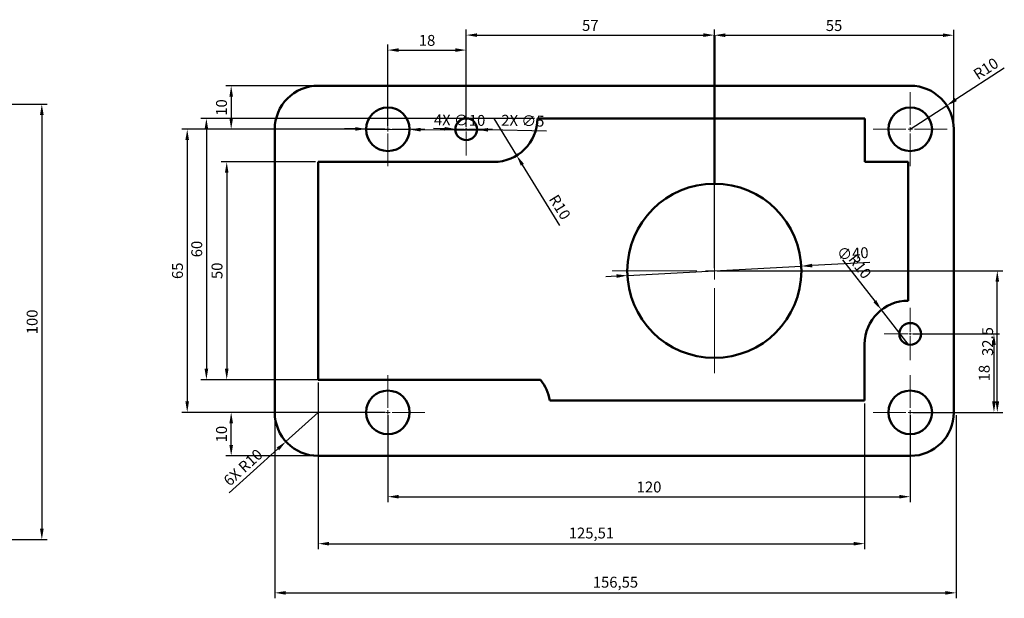
# Model space of a CAD drawing. Units: millimetres. Extents: x 1381 to 2009, y 1325 to 1613.
# Tile 4 of 6: x 1620 to 1846, y 1336 to 1469. Entities that reach past the tile are written whole.
import ezdxf

# ---------------------------------------------------------------- set-up
doc = ezdxf.new("R2010")
doc.units = ezdxf.units.MM
doc.linetypes.add('CENTER', pattern=[50.8, 31.75, -6.35, 6.35, -6.35])
for name, color, linetype, lineweight in [('M-CNTR', 1, 'CENTER', 18), ('M-DIMS', 2, 'Continuous', 25), ('M-OUTL', 7, 'Continuous', 50)]:
    doc.layers.add(name, color=color, linetype=linetype, lineweight=lineweight)
doc.styles.get("Standard").update_dxf_attribs({"font": 'arial.ttf'})
doc.dimstyles.new('ISO-25', dxfattribs={"dimtxt": 2.5, "dimasz": 2.5, "dimexe": 1.25, "dimexo": 0.625, "dimtad": 1, "dimtxsty": 'Standard', "dimcen": 2.5, "dimadec": 0, "dimazin": 0, "dimtfac": 1, "dimtmove": 0, "dimatfit": 3, "dimfxl": 1, "dimarcsym": 0})

# ---------------------------------------------------------------- blocks, each defined once
blk = doc.blocks.new('*D12')
at = {"layer": 'Defpoints', "color": 0, "transparency": 16777216}
for p in [(1722.14, 1462.15), (1704.14, 1443.96), (1722.14, 1443.96)]:
    blk.add_point(p, dxfattribs=at)
at = {"layer": 'M-DIMS', "color": 0, "lineweight": -2, "transparency": 16777216}
for p, q in [((1704.14, 1444.58), (1704.14, 1463.4)), ((1706.64, 1462.15), (1719.64, 1462.15)), ((1722.14, 1444.58), (1722.14, 1463.4))]:
    blk.add_line(p, q, dxfattribs=at)
at = {"layer": 'M-DIMS', "color": 0, "transparency": 16777216}
for points in [[(1706.64, 1462.56), (1706.64, 1461.73), (1704.14, 1462.15)], [(1719.64, 1462.56), (1719.64, 1461.73), (1722.14, 1462.15)]]:
    blk.add_solid(points, dxfattribs=at)
at = {"layer": 'M-DIMS', "color": 0, "transparency": 16777216, "insert": (1713.14, 1464.05), "char_height": 2.5, "attachment_point": 5}
blk.add_mtext('18', dxfattribs=at)
blk = doc.blocks.new('*D13')
at = {"layer": 'Defpoints', "color": 0, "transparency": 16777216}
for p in [(1779.14, 1465.59), (1722.14, 1443.96), (1779.14, 1411.46)]:
    blk.add_point(p, dxfattribs=at)
at = {"layer": 'M-DIMS', "color": 0, "lineweight": -2, "transparency": 16777216}
for p, q in [((1722.14, 1444.58), (1722.14, 1466.84)), ((1779.14, 1412.08), (1779.14, 1466.84)), ((1724.64, 1465.59), (1776.64, 1465.59))]:
    blk.add_line(p, q, dxfattribs=at)
at = {"layer": 'M-DIMS', "color": 0, "transparency": 16777216}
for points in [[(1724.64, 1466), (1724.64, 1465.17), (1722.14, 1465.59)], [(1776.64, 1466), (1776.64, 1465.17), (1779.14, 1465.59)]]:
    blk.add_solid(points, dxfattribs=at)
at = {"layer": 'M-DIMS', "color": 0, "transparency": 16777216, "insert": (1750.64, 1467.48), "char_height": 2.5, "attachment_point": 5}
blk.add_mtext('57', dxfattribs=at)
blk = doc.blocks.new('*D14')
at = {"layer": 'Defpoints', "color": 0, "transparency": 16777216}
for p in [(1834.14, 1465.56), (1834.14, 1443.96), (1779.14, 1439.46)]:
    blk.add_point(p, dxfattribs=at)
at = {"layer": 'M-DIMS', "color": 0, "lineweight": -2, "transparency": 16777216}
for p, q in [((1779.14, 1440.08), (1779.14, 1466.81)), ((1834.14, 1444.58), (1834.14, 1466.81)), ((1781.64, 1465.56), (1831.64, 1465.56))]:
    blk.add_line(p, q, dxfattribs=at)
at = {"layer": 'M-DIMS', "color": 0, "transparency": 16777216}
for points in [[(1781.64, 1465.97), (1781.64, 1465.14), (1779.14, 1465.56)], [(1831.64, 1465.97), (1831.64, 1465.14), (1834.14, 1465.56)]]:
    blk.add_solid(points, dxfattribs=at)
at = {"layer": 'M-DIMS', "color": 0, "transparency": 16777216, "insert": (1806.64, 1467.45), "char_height": 2.5, "attachment_point": 5}
blk.add_mtext('55', dxfattribs=at)
blk = doc.blocks.new('*D15')
at = {"layer": 'Defpoints', "color": 0, "transparency": 16777216}
for p in [(1824.14, 1396.96), (1824.14, 1378.96), (1843.37, 1378.96)]:
    blk.add_point(p, dxfattribs=at)
at = {"layer": 'M-DIMS', "color": 0, "lineweight": -2, "transparency": 16777216}
for p, q in [((1824.77, 1396.96), (1844.62, 1396.96)), ((1843.37, 1394.46), (1843.37, 1381.46)), ((1824.77, 1378.96), (1844.62, 1378.96))]:
    blk.add_line(p, q, dxfattribs=at)
at = {"layer": 'M-DIMS', "color": 0, "transparency": 16777216}
for points in [[(1842.95, 1394.46), (1843.79, 1394.46), (1843.37, 1396.96)], [(1842.95, 1381.46), (1843.79, 1381.46), (1843.37, 1378.96)]]:
    blk.add_solid(points, dxfattribs=at)
at = {"layer": 'M-DIMS', "color": 0, "transparency": 16777216, "insert": (1841.47, 1387.96), "char_height": 2.5, "attachment_point": 5, "rotation": 90}
blk.add_mtext('18', dxfattribs=at)
blk = doc.blocks.new('*D16')
at = {"layer": 'Defpoints', "color": 0, "transparency": 16777216}
for p in [(1678.14, 1378.96), (1834.69, 1378.96), (1834.69, 1337.51)]:
    blk.add_point(p, dxfattribs=at)
at = {"layer": 'M-DIMS', "color": 0, "lineweight": -2, "transparency": 16777216}
for p, q in [((1678.14, 1378.33), (1678.14, 1336.26)), ((1834.69, 1378.33), (1834.69, 1336.26)), ((1680.64, 1337.51), (1832.19, 1337.51))]:
    blk.add_line(p, q, dxfattribs=at)
at = {"layer": 'M-DIMS', "color": 0, "transparency": 16777216}
for points in [[(1680.64, 1337.92), (1680.64, 1337.09), (1678.14, 1337.51)], [(1832.19, 1337.92), (1832.19, 1337.09), (1834.69, 1337.51)]]:
    blk.add_solid(points, dxfattribs=at)
at = {"layer": 'M-DIMS', "color": 0, "transparency": 16777216, "insert": (1756.42, 1339.63), "char_height": 2.5, "attachment_point": 5}
blk.add_mtext('156,55', dxfattribs=at)
blk = doc.blocks.new('*D17')
at = {"layer": 'Defpoints', "color": 0, "transparency": 16777216}
for p in [(1688.14, 1386.46), (1813.66, 1381.65), (1813.66, 1348.8)]:
    blk.add_point(p, dxfattribs=at)
at = {"layer": 'M-DIMS', "color": 0, "lineweight": -2, "transparency": 16777216}
for p, q in [((1688.14, 1385.83), (1688.14, 1347.55)), ((1813.66, 1381.02), (1813.66, 1347.55)), ((1690.64, 1348.8), (1811.16, 1348.8))]:
    blk.add_line(p, q, dxfattribs=at)
at = {"layer": 'M-DIMS', "color": 0, "transparency": 16777216}
for points in [[(1690.64, 1349.21), (1690.64, 1348.38), (1688.14, 1348.8)], [(1811.16, 1349.21), (1811.16, 1348.38), (1813.66, 1348.8)]]:
    blk.add_solid(points, dxfattribs=at)
at = {"layer": 'M-DIMS', "color": 0, "transparency": 16777216, "insert": (1750.9, 1350.92), "char_height": 2.5, "attachment_point": 5}
blk.add_mtext('125,51', dxfattribs=at)
blk = doc.blocks.new('*D18')
at = {"layer": 'Defpoints', "color": 0, "transparency": 16777216}
for p in [(1704.14, 1378.96), (1824.14, 1378.96), (1824.14, 1359.59)]:
    blk.add_point(p, dxfattribs=at)
at = {"layer": 'M-DIMS', "color": 0, "lineweight": -2, "transparency": 16777216}
for p, q in [((1704.14, 1378.33), (1704.14, 1358.34)), ((1824.14, 1378.33), (1824.14, 1358.34)), ((1706.64, 1359.59), (1821.64, 1359.59))]:
    blk.add_line(p, q, dxfattribs=at)
at = {"layer": 'M-DIMS', "color": 0, "transparency": 16777216}
for points in [[(1706.64, 1360), (1706.64, 1359.17), (1704.14, 1359.59)], [(1821.64, 1360), (1821.64, 1359.17), (1824.14, 1359.59)]]:
    blk.add_solid(points, dxfattribs=at)
at = {"layer": 'M-DIMS', "color": 0, "transparency": 16777216, "insert": (1764.14, 1361.49), "char_height": 2.5, "attachment_point": 5}
blk.add_mtext('120', dxfattribs=at)
blk = doc.blocks.new('*D19')
at = {"layer": 'Defpoints', "color": 0, "transparency": 16777216}
for p in [(1832.53, 1449.4), (1824.14, 1443.96)]:
    blk.add_point(p, dxfattribs=at)
at = {"layer": 'M-DIMS', "color": 0, "lineweight": -2, "transparency": 16777216}
for p, q in [((1845.75, 1457.99), (1834.63, 1450.77)), ((1824.14, 1443.96), (1832.53, 1449.4))]:
    blk.add_line(p, q, dxfattribs=at)
at = {"layer": 'M-DIMS', "color": 0, "transparency": 16777216}
blk.add_solid([(1834.4, 1451.12), (1834.85, 1450.42), (1832.53, 1449.4)], dxfattribs=at)
at = {"layer": 'M-DIMS', "color": 0, "transparency": 16777216, "insert": (1841.69, 1457.62), "char_height": 2.5, "attachment_point": 5, "rotation": 32.9978}
blk.add_mtext('R10', dxfattribs=at)
blk = doc.blocks.new('*D20')
at = {"layer": 'Defpoints', "color": 0, "transparency": 16777216}
for p in [(1728.48, 1446.46), (1733.72, 1437.95)]:
    blk.add_point(p, dxfattribs=at)
at = {"layer": 'M-DIMS', "color": 0, "lineweight": -2, "transparency": 16777216}
for p, q in [((1728.48, 1446.46), (1733.72, 1437.95)), ((1743.65, 1421.84), (1735.04, 1435.82))]:
    blk.add_line(p, q, dxfattribs=at)
at = {"layer": 'M-DIMS', "color": 0, "transparency": 16777216}
blk.add_solid([(1735.39, 1436.04), (1734.68, 1435.6), (1733.72, 1437.95)], dxfattribs=at)
at = {"layer": 'M-DIMS', "color": 0, "transparency": 16777216, "insert": (1743.38, 1425.91), "char_height": 2.5, "attachment_point": 5, "rotation": 301.6495}
blk.add_mtext('R10', dxfattribs=at)
blk = doc.blocks.new('*D21')
at = {"layer": 'Defpoints', "color": 0, "transparency": 16777216}
for p in [(1817.52, 1402.5), (1823.66, 1394.6)]:
    blk.add_point(p, dxfattribs=at)
at = {"layer": 'M-DIMS', "color": 0, "lineweight": -2, "transparency": 16777216}
for p, q in [((1808.61, 1413.95), (1815.99, 1404.47)), ((1823.66, 1394.6), (1817.52, 1402.5))]:
    blk.add_line(p, q, dxfattribs=at)
at = {"layer": 'M-DIMS', "color": 0, "transparency": 16777216}
blk.add_solid([(1816.32, 1404.73), (1815.66, 1404.22), (1817.52, 1402.5)], dxfattribs=at)
at = {"layer": 'M-DIMS', "color": 0, "transparency": 16777216, "insert": (1812.33, 1412.27), "char_height": 2.5, "attachment_point": 5, "rotation": 307.8622}
blk.add_mtext('R10', dxfattribs=at)
blk = doc.blocks.new('*U22')
at = {"layer": 'M-CNTR', "color": 0, "transparency": 16777216}
for p, q in [((0, 4), (0, 23.5)), ((-23.5, 0), (-4, 0)), ((4, 0), (23.5, 0)), ((0, -23.5), (0, -4))]:
    blk.add_line(p, q, dxfattribs=at)
at = {"layer": 'M-CNTR', "color": 0, "linetype": 'Continuous', "transparency": 16777216}
for p, q in [((-2, 0), (2, 0)), ((0, -2), (0, 2))]:
    blk.add_line(p, q, dxfattribs=at)
blk = doc.blocks.new('*U23')
at = {"layer": 'M-CNTR', "color": 0, "transparency": 16777216}
for p, q in [((0, 1), (0, 8.5)), ((-8.5, 0), (-1, 0)), ((1, 0), (8.5, 0)), ((0, -8.5), (0, -1))]:
    blk.add_line(p, q, dxfattribs=at)
at = {"layer": 'M-CNTR', "color": 0, "linetype": 'Continuous', "transparency": 16777216}
for p, q in [((-0.5, 0), (0.5, 0)), ((0, -0.5), (0, 0.5))]:
    blk.add_line(p, q, dxfattribs=at)
blk = doc.blocks.new('*U24')
at = {"layer": 'M-CNTR', "color": 0, "transparency": 16777216}
for p, q in [((0, 0.5), (0, 6)), ((-6, 0), (-0.5, 0)), ((0.5, 0), (6, 0)), ((0, -6), (0, -0.5))]:
    blk.add_line(p, q, dxfattribs=at)
at = {"layer": 'M-CNTR', "color": 0, "linetype": 'Continuous', "transparency": 16777216}
for p, q in [((-0.25, 0), (0.25, 0)), ((0, -0.25), (0, 0.25))]:
    blk.add_line(p, q, dxfattribs=at)
blk = doc.blocks.new('*U25')
at = {"layer": 'M-CNTR', "color": 0, "transparency": 16777216}
for p, q in [((0, 1), (0, 8.5)), ((-8.5, 0), (-1, 0)), ((1, 0), (8.5, 0)), ((0, -8.5), (0, -1))]:
    blk.add_line(p, q, dxfattribs=at)
at = {"layer": 'M-CNTR', "color": 0, "linetype": 'Continuous', "transparency": 16777216}
for p, q in [((-0.5, 0), (0.5, 0)), ((0, -0.5), (0, 0.5))]:
    blk.add_line(p, q, dxfattribs=at)
blk = doc.blocks.new('*U26')
at = {"layer": 'M-CNTR', "color": 0, "transparency": 16777216}
for p, q in [((0, 1), (0, 8.5)), ((-8.5, 0), (-1, 0)), ((1, 0), (8.5, 0)), ((0, -8.5), (0, -1))]:
    blk.add_line(p, q, dxfattribs=at)
at = {"layer": 'M-CNTR', "color": 0, "linetype": 'Continuous', "transparency": 16777216}
for p, q in [((-0.5, 0), (0.5, 0)), ((0, -0.5), (0, 0.5))]:
    blk.add_line(p, q, dxfattribs=at)
blk = doc.blocks.new('*U27')
at = {"layer": 'M-CNTR', "color": 0, "transparency": 16777216}
for p, q in [((0, 0.5), (0, 6)), ((-6, 0), (-0.5, 0)), ((0.5, 0), (6, 0)), ((0, -6), (0, -0.5))]:
    blk.add_line(p, q, dxfattribs=at)
at = {"layer": 'M-CNTR', "color": 0, "linetype": 'Continuous', "transparency": 16777216}
for p, q in [((-0.25, 0), (0.25, 0)), ((0, -0.25), (0, 0.25))]:
    blk.add_line(p, q, dxfattribs=at)
blk = doc.blocks.new('*U28')
at = {"layer": 'M-CNTR', "color": 0, "transparency": 16777216}
for p, q in [((0, 1), (0, 8.5)), ((-8.5, 0), (-1, 0)), ((1, 0), (8.5, 0)), ((0, -8.5), (0, -1))]:
    blk.add_line(p, q, dxfattribs=at)
at = {"layer": 'M-CNTR', "color": 0, "linetype": 'Continuous', "transparency": 16777216}
for p, q in [((-0.5, 0), (0.5, 0)), ((0, -0.5), (0, 0.5))]:
    blk.add_line(p, q, dxfattribs=at)
blk = doc.blocks.new('*D29')
at = {"layer": 'Defpoints', "color": 0, "transparency": 16777216}
for p in [(1704.14, 1443.96), (1658.04, 1378.96), (1704.14, 1378.96)]:
    blk.add_point(p, dxfattribs=at)
at = {"layer": 'M-DIMS', "color": 0, "lineweight": -2, "transparency": 16777216}
for p, q in [((1703.52, 1443.96), (1656.79, 1443.96)), ((1658.04, 1441.46), (1658.04, 1381.46)), ((1703.52, 1378.96), (1656.79, 1378.96))]:
    blk.add_line(p, q, dxfattribs=at)
at = {"layer": 'M-DIMS', "color": 0, "transparency": 16777216}
for points in [[(1657.62, 1441.46), (1658.45, 1441.46), (1658.04, 1443.96)], [(1657.62, 1381.46), (1658.45, 1381.46), (1658.04, 1378.96)]]:
    blk.add_solid(points, dxfattribs=at)
at = {"layer": 'M-DIMS', "color": 0, "transparency": 16777216, "insert": (1656.13, 1411.46), "char_height": 2.5, "attachment_point": 5, "rotation": 90}
blk.add_mtext('65', dxfattribs=at)
blk = doc.blocks.new('*D30')
at = {"layer": 'Defpoints', "color": 0, "transparency": 16777216}
for p in [(1688.14, 1436.46), (1667.12, 1386.46), (1688.14, 1386.46)]:
    blk.add_point(p, dxfattribs=at)
at = {"layer": 'M-DIMS', "color": 0, "lineweight": -2, "transparency": 16777216}
for p, q in [((1687.52, 1436.46), (1665.87, 1436.46)), ((1667.12, 1433.96), (1667.12, 1388.96)), ((1687.52, 1386.46), (1665.87, 1386.46))]:
    blk.add_line(p, q, dxfattribs=at)
at = {"layer": 'M-DIMS', "color": 0, "transparency": 16777216}
for points in [[(1666.7, 1433.96), (1667.53, 1433.96), (1667.12, 1436.46)], [(1666.7, 1388.96), (1667.53, 1388.96), (1667.12, 1386.46)]]:
    blk.add_solid(points, dxfattribs=at)
at = {"layer": 'M-DIMS', "color": 0, "transparency": 16777216, "insert": (1665.21, 1411.46), "char_height": 2.5, "attachment_point": 5, "rotation": 90}
blk.add_mtext('50', dxfattribs=at)
blk = doc.blocks.new('*D31')
at = {"layer": 'Defpoints', "color": 0, "transparency": 16777216}
for p in [(1738.48, 1446.46), (1662.45, 1386.46), (1739.2, 1386.46)]:
    blk.add_point(p, dxfattribs=at)
at = {"layer": 'M-DIMS', "color": 0, "lineweight": -2, "transparency": 16777216}
for p, q in [((1737.85, 1446.46), (1661.2, 1446.46)), ((1662.45, 1443.96), (1662.45, 1388.96)), ((1738.58, 1386.46), (1661.2, 1386.46))]:
    blk.add_line(p, q, dxfattribs=at)
at = {"layer": 'M-DIMS', "color": 0, "transparency": 16777216}
for points in [[(1662.03, 1443.96), (1662.86, 1443.96), (1662.45, 1446.46)], [(1662.03, 1388.96), (1662.86, 1388.96), (1662.45, 1386.46)]]:
    blk.add_solid(points, dxfattribs=at)
at = {"layer": 'M-DIMS', "color": 0, "transparency": 16777216, "insert": (1660.55, 1416.46), "char_height": 2.5, "attachment_point": 5, "rotation": 90}
blk.add_mtext('60', dxfattribs=at)
blk = doc.blocks.new('*D39')
at = {"layer": 'Defpoints', "color": 0, "transparency": 16777216}
for p in [(1600.47, 1449.73), (1600.47, 1349.73), (1624.64, 1349.73)]:
    blk.add_point(p, dxfattribs=at)
at = {"layer": 'M-DIMS', "color": 0, "lineweight": -2, "transparency": 16777216}
for p, q in [((1601.1, 1449.73), (1625.89, 1449.73)), ((1624.64, 1447.23), (1624.64, 1352.23)), ((1601.1, 1349.73), (1625.89, 1349.73))]:
    blk.add_line(p, q, dxfattribs=at)
at = {"layer": 'M-DIMS', "color": 0, "transparency": 16777216}
for points in [[(1624.22, 1447.23), (1625.06, 1447.23), (1624.64, 1449.73)], [(1624.22, 1352.23), (1625.06, 1352.23), (1624.64, 1349.73)]]:
    blk.add_solid(points, dxfattribs=at)
at = {"layer": 'M-DIMS', "color": 0, "transparency": 16777216, "insert": (1622.74, 1399.73), "char_height": 2.5, "attachment_point": 5, "rotation": 90}
blk.add_mtext('100', dxfattribs=at)
blk = doc.blocks.new('*D97')
at = {"layer": 'Defpoints', "color": 0, "transparency": 16777216}
for p in [(1688.14, 1453.96), (1668.14, 1443.96), (1704.14, 1443.96)]:
    blk.add_point(p, dxfattribs=at)
at = {"layer": 'M-DIMS', "color": 0, "lineweight": -2, "transparency": 16777216}
for p, q in [((1687.52, 1453.96), (1666.89, 1453.96)), ((1668.14, 1451.46), (1668.14, 1446.46)), ((1703.52, 1443.96), (1666.89, 1443.96))]:
    blk.add_line(p, q, dxfattribs=at)
at = {"layer": 'M-DIMS', "color": 0, "transparency": 16777216}
for points in [[(1667.73, 1451.46), (1668.56, 1451.46), (1668.14, 1453.96)], [(1667.73, 1446.46), (1668.56, 1446.46), (1668.14, 1443.96)]]:
    blk.add_solid(points, dxfattribs=at)
at = {"layer": 'M-DIMS', "color": 0, "transparency": 16777216, "insert": (1666.24, 1448.96), "char_height": 2.5, "attachment_point": 5, "rotation": 90}
blk.add_mtext('10', dxfattribs=at)
blk = doc.blocks.new('*D98')
at = {"layer": 'Defpoints', "color": 0, "transparency": 16777216}
for p in [(1668.14, 1378.96), (1704.14, 1378.96), (1688.14, 1368.96)]:
    blk.add_point(p, dxfattribs=at)
at = {"layer": 'M-DIMS', "color": 0, "lineweight": -2, "transparency": 16777216}
for p, q in [((1703.52, 1378.96), (1666.89, 1378.96)), ((1668.14, 1371.46), (1668.14, 1376.46)), ((1687.52, 1368.96), (1666.89, 1368.96))]:
    blk.add_line(p, q, dxfattribs=at)
at = {"layer": 'M-DIMS', "color": 0, "transparency": 16777216}
for points in [[(1667.73, 1376.46), (1668.56, 1376.46), (1668.14, 1378.96)], [(1667.73, 1371.46), (1668.56, 1371.46), (1668.14, 1368.96)]]:
    blk.add_solid(points, dxfattribs=at)
at = {"layer": 'M-DIMS', "color": 0, "transparency": 16777216, "insert": (1666.24, 1373.96), "char_height": 2.5, "attachment_point": 5, "rotation": 90}
blk.add_mtext('10', dxfattribs=at)
blk = doc.blocks.new('*D99')
at = {"layer": 'Defpoints', "color": 0, "transparency": 16777216}
for p in [(1779.14, 1411.46), (1844.14, 1411.46), (1824.64, 1378.96)]:
    blk.add_point(p, dxfattribs=at)
at = {"layer": 'M-DIMS', "color": 0, "lineweight": -2, "transparency": 16777216}
for p, q in [((1779.77, 1411.46), (1845.39, 1411.46)), ((1844.14, 1381.46), (1844.14, 1408.96)), ((1825.27, 1378.96), (1845.39, 1378.96))]:
    blk.add_line(p, q, dxfattribs=at)
at = {"layer": 'M-DIMS', "color": 0, "transparency": 16777216}
for points in [[(1843.73, 1408.96), (1844.56, 1408.96), (1844.14, 1411.46)], [(1843.73, 1381.46), (1844.56, 1381.46), (1844.14, 1378.96)]]:
    blk.add_solid(points, dxfattribs=at)
at = {"layer": 'M-DIMS', "color": 0, "transparency": 16777216, "insert": (1842.24, 1395.21), "char_height": 2.5, "attachment_point": 5, "rotation": 90}
blk.add_mtext('32.5', dxfattribs=at)
blk = doc.blocks.new('*D126')
at = {"layer": 'Defpoints', "color": 0, "transparency": 16777216}
for p in [(1699.14, 1444.02), (1709.14, 1443.9)]:
    blk.add_point(p, dxfattribs=at)
at = {"layer": 'M-DIMS', "color": 0, "lineweight": -2, "transparency": 16777216}
for p, q in [((1696.64, 1444.05), (1694.14, 1444.08)), ((1699.14, 1444.02), (1709.14, 1443.9)), ((1727.02, 1443.68), (1711.64, 1443.87))]:
    blk.add_line(p, q, dxfattribs=at)
at = {"layer": 'M-DIMS', "color": 0, "transparency": 16777216}
for points in [[(1696.65, 1444.46), (1696.64, 1443.63), (1699.14, 1444.02)], [(1711.65, 1444.29), (1711.64, 1443.45), (1709.14, 1443.9)]]:
    blk.add_solid(points, dxfattribs=at)
at = {"layer": 'M-DIMS', "color": 0, "transparency": 16777216, "insert": (1720.61, 1445.73), "char_height": 2.5, "attachment_point": 5, "rotation": 359.3156}
blk.add_mtext('4X ∅10', dxfattribs=at)
blk = doc.blocks.new('*D127')
at = {"layer": 'Defpoints', "color": 0, "transparency": 16777216}
for p in [(1719.64, 1444.02), (1724.64, 1443.9)]:
    blk.add_point(p, dxfattribs=at)
at = {"layer": 'M-DIMS', "color": 0, "lineweight": -2, "transparency": 16777216}
for p, q in [((1717.15, 1444.08), (1714.65, 1444.14)), ((1719.64, 1444.02), (1724.64, 1443.9)), ((1740.55, 1443.5), (1727.14, 1443.83))]:
    blk.add_line(p, q, dxfattribs=at)
at = {"layer": 'M-DIMS', "color": 0, "transparency": 16777216}
for points in [[(1717.16, 1444.5), (1717.13, 1443.66), (1719.64, 1444.02)], [(1727.15, 1444.25), (1727.13, 1443.42), (1724.64, 1443.9)]]:
    blk.add_solid(points, dxfattribs=at)
at = {"layer": 'M-DIMS', "color": 0, "transparency": 16777216, "insert": (1735.14, 1445.61), "char_height": 2.5, "attachment_point": 5, "rotation": 358.5897}
blk.add_mtext('2X ∅5', dxfattribs=at)
blk = doc.blocks.new('*D128')
at = {"layer": 'Defpoints', "color": 0, "transparency": 16777216}
for p in [(1799.11, 1412.53), (1759.17, 1410.38)]:
    blk.add_point(p, dxfattribs=at)
at = {"layer": 'M-DIMS', "color": 0, "lineweight": -2, "transparency": 16777216}
for p, q in [((1759.17, 1410.38), (1799.11, 1412.53)), ((1814.86, 1413.38), (1801.61, 1412.67)), ((1756.68, 1410.25), (1754.18, 1410.11))]:
    blk.add_line(p, q, dxfattribs=at)
at = {"layer": 'M-DIMS', "color": 0, "transparency": 16777216}
for points in [[(1801.59, 1413.08), (1801.63, 1412.25), (1799.11, 1412.53)], [(1756.65, 1410.66), (1756.7, 1409.83), (1759.17, 1410.38)]]:
    blk.add_solid(points, dxfattribs=at)
at = {"layer": 'M-DIMS', "color": 0, "transparency": 16777216, "insert": (1810.99, 1415.15), "char_height": 2.5, "attachment_point": 5, "rotation": 3.0814}
blk.add_mtext('∅40', dxfattribs=at)
blk = doc.blocks.new('*D129')
at = {"layer": 'Defpoints', "color": 0, "transparency": 16777216}
for p in [(1688.14, 1378.96), (1680.73, 1372.25)]:
    blk.add_point(p, dxfattribs=at)
at = {"layer": 'M-DIMS', "color": 0, "lineweight": -2, "transparency": 16777216}
for p, q in [((1688.14, 1378.96), (1680.73, 1372.25)), ((1667.68, 1360.44), (1678.88, 1370.57))]:
    blk.add_line(p, q, dxfattribs=at)
at = {"layer": 'M-DIMS', "color": 0, "transparency": 16777216}
blk.add_solid([(1678.6, 1370.88), (1679.16, 1370.26), (1680.73, 1372.25)], dxfattribs=at)
at = {"layer": 'M-DIMS', "color": 0, "transparency": 16777216, "insert": (1671.08, 1366.07), "char_height": 2.5, "attachment_point": 5, "rotation": 42.1526}
blk.add_mtext('6X R10', dxfattribs=at)

msp = doc.modelspace()

# ---------------------------------------------------------------- linework, layer by layer
at = {"layer": 'M-OUTL'}
for p, q in [((1779.1437, 1431.458), (1779.1437, 1465.5862)), ((1688.1437, 1453.958), (1824.1437, 1453.958)), ((1738.4764, 1446.458), (1738.4764, 1446.458)), ((1738.4764, 1446.458), (1813.7365, 1446.458)), ((1813.7365, 1446.458), (1813.7365, 1436.458)), ((1678.1437, 1378.958), (1678.1437, 1443.958)), ((1834.1437, 1443.958), (1834.1437, 1378.958)), ((1688.1437, 1411.458), (1688.1437, 1436.458)), ((1688.1437, 1436.458), (1728.4764, 1436.458)), ((1813.7365, 1436.458), (1823.6583, 1436.458)), ((1823.6583, 1436.458), (1823.6583, 1404.6026)), ((1688.1437, 1411.458), (1688.1437, 1386.458)), ((1823.6583, 1404.6026), (1823.6583, 1404.6026)), ((1813.6583, 1394.6026), (1813.6583, 1381.6454)), ((1688.1437, 1386.458), (1739.2024, 1386.458)), ((1813.6583, 1381.6454), (1741.3162, 1381.6454)), ((1824.1437, 1368.958), (1688.1437, 1368.958))]:
    msp.add_line(p, q, dxfattribs=at)
for centre, radius in [((1704.1437, 1443.958), 5), ((1824.1437, 1443.958), 5), ((1722.1437, 1443.958), 2.5), ((1779.1437, 1411.458), 20), ((1824.1437, 1396.958), 2.5), ((1704.1437, 1378.958), 5), ((1824.1437, 1378.958), 5)]:
    msp.add_circle(centre, radius, dxfattribs=at)
for centre, start, end in [((1688.1437, 1443.958), 90, 180), ((1824.1437, 1443.958), 0, 90), ((1728.4764, 1446.458), 270, 0), ((1823.6583, 1394.6026), 90, 180), ((1731.4254, 1380.1716), 8.475265, 38.949946), ((1688.1437, 1378.958), 180, 270), ((1824.1437, 1378.958), 270, 0)]:
    msp.add_arc(centre, 10, start, end, dxfattribs=at)

# ---------------------------------------------------------------- block references
at = {"layer": 'M-CNTR'}
for name, p in [('*U23', (1704.1437, 1443.958)), ('*U28', (1824.1437, 1443.958)), ('*U24', (1722.1437, 1443.958)), ('*U22', (1779.1437, 1411.458)), ('*U27', (1824.1437, 1396.958)), ('*U25', (1704.1437, 1378.958)), ('*U26', (1824.1437, 1378.958))]:
    msp.add_blockref(name, p, dxfattribs=at)

# ---------------------------------------------------------------- dimensions: what is measured, and where the dimension line sits
at = {"layer": 'M-DIMS'}
for base, p1, p2, picture, middle in [((1779.1437, 1465.5862), (1722.1437, 1443.958), (1779.1437, 1411.458), '*D13', (1750.6437, 1467.4825)), ((1834.1437, 1465.5558), (1779.1437, 1439.4596), (1834.1437, 1443.958), '*D14', (1806.6437, 1467.4521)), ((1722.1437, 1462.1479), (1704.1437, 1443.958), (1722.1437, 1443.958), '*D12', (1713.1437, 1464.0493)), ((1813.6583, 1348.7976), (1688.1437, 1386.458), (1813.6583, 1381.6454), '*D17', (1750.901, 1350.925)), ((1834.694, 1337.5054), (1678.1437, 1378.958), (1834.694, 1378.958), '*D16', (1756.4188, 1339.6328)), ((1824.1437, 1359.5879), (1704.1437, 1378.958), (1824.1437, 1378.958), '*D18', (1764.1437, 1361.4893))]:
    dim = msp.add_linear_dim(base=base, p1=p1, p2=p2, dimstyle='ISO-25', override={"dimclrd": 0, "dimclre": 0, "dimclrt": 0}, dxfattribs=at)
    dim.commit()
    dim.dimension.update_dxf_attribs({"geometry": picture, "text_midpoint": middle})
for center, mpoint, picture, middle in [((1824.1437, 1443.958), (1832.5306, 1449.4041), '*D19', (1842.7251, 1456.0239)), ((1728.4764, 1446.458), (1733.7236, 1437.9453), '*D20', (1741.76, 1424.9076)), ((1823.6583, 1394.6026), (1817.5206, 1402.4975), '*D21', (1810.8282, 1411.1061))]:
    dim = msp.add_radius_dim(center=center, mpoint=mpoint, dimstyle='ISO-25', override={"dimclrd": 0, "dimclre": 0, "dimclrt": 0}, dxfattribs=at)
    dim.commit()
    dim.dimension.update_dxf_attribs({"geometry": picture, "text_midpoint": middle, "dimtype": 164})
for base, p1, p2, override, picture, middle in [((1668.1437, 1443.958), (1688.1437, 1453.958), (1704.1437, 1443.958), {"dimdec": 0, "dimlfac": 1, "dimrnd": 0, "dimzin": 0, "dimdsep": 46, "dimlunit": 2}, '*D97', (1666.2423, 1448.958)), ((1624.6414, 1349.7301), (1600.4722, 1449.7301), (1600.4722, 1349.7301), {"dimclrd": 0, "dimclre": 0, "dimclrt": 0}, '*D39', (1622.74, 1399.7301)), ((1662.4465, 1386.458), (1738.4764, 1446.458), (1739.2024, 1386.458), {"dimclrd": 0, "dimclre": 0, "dimclrt": 0}, '*D31', (1660.5451, 1416.458)), ((1658.0361, 1378.958), (1704.1437, 1443.958), (1704.1437, 1378.958), {"dimclrd": 0, "dimclre": 0, "dimclrt": 0}, '*D29', (1656.1346, 1411.458)), ((1667.1157, 1386.458), (1688.1437, 1436.458), (1688.1437, 1386.458), {"dimclrd": 0, "dimclre": 0, "dimclrt": 0}, '*D30', (1665.2143, 1411.458)), ((1844.1437, 1411.458), (1824.6437, 1378.958), (1779.1437, 1411.458), {"dimdec": 1, "dimlfac": 1, "dimrnd": 0, "dimzin": 0, "dimdsep": 46, "dimlunit": 2}, '*D99', (1842.2414, 1395.208)), ((1843.3692, 1378.958), (1824.1437, 1396.958), (1824.1437, 1378.958), {"dimclrd": 0, "dimclre": 0, "dimclrt": 0}, '*D15', (1841.4678, 1387.958)), ((1668.1437, 1378.958), (1688.1437, 1368.958), (1704.1437, 1378.958), {"dimdec": 0, "dimlfac": 1, "dimrnd": 0, "dimzin": 0, "dimdsep": 46, "dimlunit": 2}, '*D98', (1666.2423, 1373.958))]:
    dim = msp.add_linear_dim(base=base, p1=p1, p2=p2, angle=90, dimstyle='ISO-25', override=override, dxfattribs=at)
    dim.commit()
    dim.dimension.update_dxf_attribs({"geometry": picture, "text_midpoint": middle})
for p1, p2, text, picture, middle in [((1699.1441, 1444.0177), (1709.1434, 1443.8983), '4X <>', '*D126', (1720.5835, 1443.7616)), ((1719.6445, 1444.0195), (1724.643, 1443.8965), '2X <>', '*D127', (1735.0943, 1443.6392))]:
    dim = msp.add_diameter_dim_2p(p1=p1, p2=p2, text=text, dimstyle='ISO-25', override={"dimdec": 0, "dimlfac": 1, "dimrnd": 0, "dimzin": 0, "dimdsep": 46, "dimlunit": 2}, dxfattribs=at)
    dim.commit()
    dim.dimension.update_dxf_attribs({"geometry": picture, "text_midpoint": middle, "dimtype": 163})
dim = msp.add_diameter_dim_2p(p1=(1759.1726, 1410.3829), p2=(1799.1148, 1412.5331), dimstyle='ISO-25', override={"dimdec": 0, "dimlfac": 1, "dimrnd": 0, "dimzin": 0, "dimdsep": 46, "dimlunit": 2}, dxfattribs=at)
dim.commit()
dim.dimension.update_dxf_attribs({"geometry": '*D128', "text_midpoint": (1811.0974, 1413.1781), "dimtype": 163})
dim = msp.add_radius_dim(center=(1688.1437, 1378.958), mpoint=(1680.7301, 1372.2469), text='6X <>', dimstyle='ISO-25', override={"dimdec": 0, "dimlfac": 1, "dimrnd": 0, "dimzin": 0, "dimdsep": 46, "dimlunit": 2}, dxfattribs=at)
dim.commit()
dim.dimension.update_dxf_attribs({"geometry": '*D129', "text_midpoint": (1671.0764, 1366.0729)})

doc.saveas('drawing.dxf')
